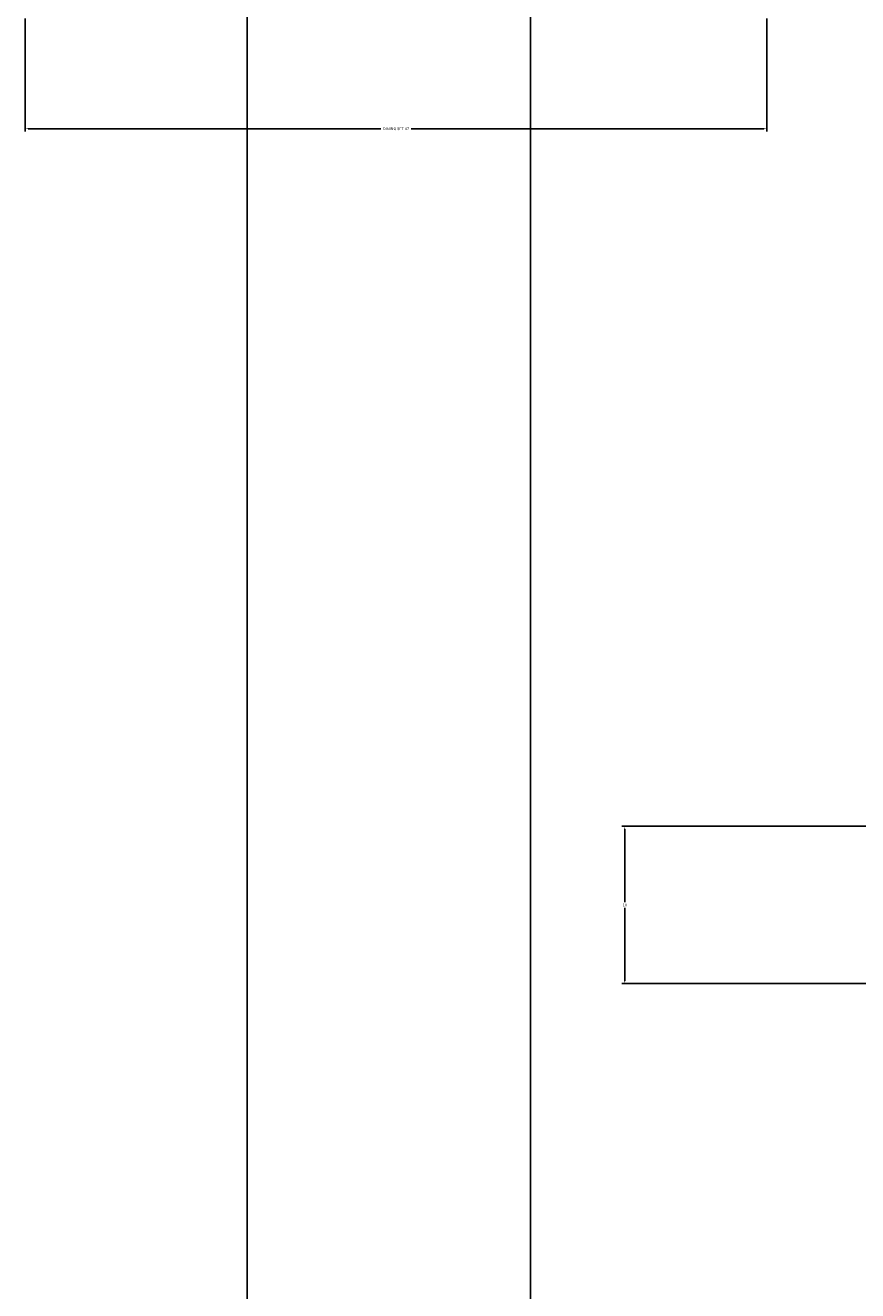
# Model space of a CAD drawing. Units: inches. Extents: x 2621 to 2849, y 2066 to 2463.
# Tile 5 of 28: x 2732 to 2785, y 2119 to 2199. Entities that reach past the tile are written whole.
import ezdxf

# ---------------------------------------------------------------- set-up
doc = ezdxf.new("R2010")
doc.units = ezdxf.units.IN
doc.layers.add('A-ANNO-DIMS', color=2, linetype='Continuous', lineweight=18)
doc.styles.get("Standard").update_dxf_attribs({"font": 'arial.ttf'})
doc.dimstyles.get("Standard").update_dxf_attribs({"dimtxt": 0.18, "dimasz": 0.18, "dimexe": 0.18, "dimexo": 0.0625, "dimgap": 0.09, "dimtad": 0, "dimtih": 1, "dimtoh": 1, "dimdec": 4, "dimzin": 0, "dimdsep": 46, "dimtxsty": 'Standard', "dimcen": 0.09, "dimadec": 0, "dimazin": 0, "dimtfac": 1, "dimtdec": 4, "dimtofl": 0, "dimtmove": 0, "dimatfit": 3, "dimfxl": 1, "dimtolj": 1, "dimtzin": 0, "dimarcsym": 0})

# ---------------------------------------------------------------- blocks, each defined once
blk = doc.blocks.new('*D25')
at = {"layer": 'A-ANNO-DIMS', "color": 0, "lineweight": -2, "transparency": 16777216}
for p, q in [((2731.763, 2199.807), (2731.763, 2192.62)), ((2778.896, 2199.807), (2778.896, 2192.62)), ((2731.943, 2192.8), (2754.36, 2192.8)), ((2778.716, 2192.8), (2756.298, 2192.8))]:
    blk.add_line(p, q, dxfattribs=at)
at = {"layer": 'A-ANNO-DIMS', "color": 0, "transparency": 16777216}
for points in [[(2731.943, 2192.83), (2731.943, 2192.77), (2731.763, 2192.8)], [(2778.716, 2192.83), (2778.716, 2192.77), (2778.896, 2192.8)]]:
    blk.add_solid(points, dxfattribs=at)
at = {"layer": 'Defpoints', "color": 0, "transparency": 16777216}
for p in [(2731.763, 2199.87), (2778.896, 2199.87), (2778.896, 2192.8)]:
    blk.add_point(p, dxfattribs=at)
at = {"layer": 'A-ANNO-DIMS', "color": 0, "transparency": 16777216, "insert": (2755.329, 2192.8), "char_height": 0.18, "attachment_point": 5}
blk.add_mtext('\\A1;DINING SET 47', dxfattribs=at)
blk = doc.blocks.new('*D61')
at = {"layer": 'A-ANNO-DIMS', "color": 0, "lineweight": -2, "transparency": 16777216}
for p, q in [((2787.808, 2148.46), (2769.687, 2148.46)), ((2769.867, 2148.28), (2769.867, 2143.642)), ((2769.867, 2138.64), (2769.867, 2143.278)), ((2787.808, 2138.46), (2769.687, 2138.46))]:
    blk.add_line(p, q, dxfattribs=at)
at = {"layer": 'A-ANNO-DIMS', "color": 0, "transparency": 16777216}
for points in [[(2769.837, 2148.28), (2769.897, 2148.28), (2769.867, 2148.46)], [(2769.837, 2138.64), (2769.897, 2138.64), (2769.867, 2138.46)]]:
    blk.add_solid(points, dxfattribs=at)
at = {"layer": 'Defpoints', "color": 0, "transparency": 16777216}
for p in [(2769.867, 2148.46), (2787.87, 2148.46), (2787.87, 2138.46)]:
    blk.add_point(p, dxfattribs=at)
at = {"layer": 'A-ANNO-DIMS', "color": 0, "transparency": 16777216, "insert": (2769.867, 2143.46), "char_height": 0.18, "attachment_point": 5}
blk.add_mtext('\\A1;10', dxfattribs=at)
blk = doc.blocks.new('*D70')
at = {"layer": 'A-ANNO-DIMS', "color": 0, "lineweight": -2, "transparency": 16777216}
for p, q in [((2745.856, 2291.312), (2745.856, 2066.191)), ((2763.87, 2291.312), (2763.87, 2066.191)), ((2746.036, 2066.371), (2754.408, 2066.371)), ((2763.69, 2066.371), (2755.318, 2066.371))]:
    blk.add_line(p, q, dxfattribs=at)
at = {"layer": 'A-ANNO-DIMS', "color": 0, "transparency": 16777216}
for points in [[(2746.036, 2066.401), (2746.036, 2066.341), (2745.856, 2066.371)], [(2763.69, 2066.401), (2763.69, 2066.341), (2763.87, 2066.371)]]:
    blk.add_solid(points, dxfattribs=at)
at = {"layer": 'Defpoints', "color": 0, "transparency": 16777216}
for p in [(2745.856, 2291.375), (2763.87, 2291.375), (2763.87, 2066.371)]:
    blk.add_point(p, dxfattribs=at)
at = {"layer": 'A-ANNO-DIMS', "color": 0, "transparency": 16777216, "insert": (2754.863, 2066.371), "char_height": 0.18, "attachment_point": 5}
blk.add_mtext('\\A1;18.014', dxfattribs=at)

msp = doc.modelspace()

# ---------------------------------------------------------------- dimensions: what is measured, and where the dimension line sits
at = {"layer": 'A-ANNO-DIMS'}
dim = msp.add_linear_dim(base=(2763.8701, 2066.3711), p1=(2745.8562, 2291.3746), p2=(2763.8701, 2291.3746), dimstyle='Standard', override={"dimdec": 3, "dimlfac": 1, "dimrnd": 0, "dimzin": 0, "dimdsep": 46, "dimlunit": 2}, dxfattribs=at)
dim.commit()
dim.dimension.update_dxf_attribs({"geometry": '*D70', "text_midpoint": (2754.8631, 2066.3711)})
dim = msp.add_linear_dim(base=(2778.8957, 2192.7999), p1=(2731.7628, 2199.8698), p2=(2778.8957, 2199.8698), text='DINING SET <>', dimstyle='Standard', override={"dimdec": 0, "dimlfac": 1, "dimrnd": 0, "dimzin": 0, "dimdsep": 46, "dimlunit": 2}, dxfattribs=at)
dim.commit()
dim.dimension.update_dxf_attribs({"geometry": '*D25', "text_midpoint": (2755.3293, 2192.7999)})
dim = msp.add_linear_dim(base=(2769.8666, 2148.4598), p1=(2787.8701, 2138.4598), p2=(2787.8701, 2148.4598), angle=90, dimstyle='Standard', override={"dimdec": 0, "dimlfac": 1, "dimrnd": 0, "dimzin": 0, "dimdsep": 46, "dimlunit": 2}, dxfattribs=at)
dim.commit()
dim.dimension.update_dxf_attribs({"geometry": '*D61', "text_midpoint": (2769.8666, 2143.4598)})

doc.saveas('drawing.dxf')
